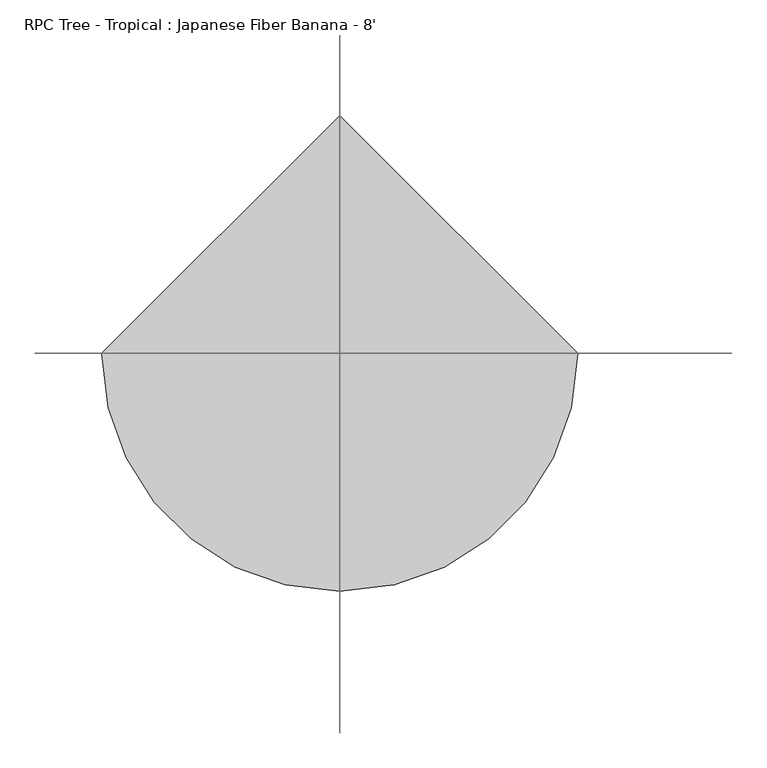
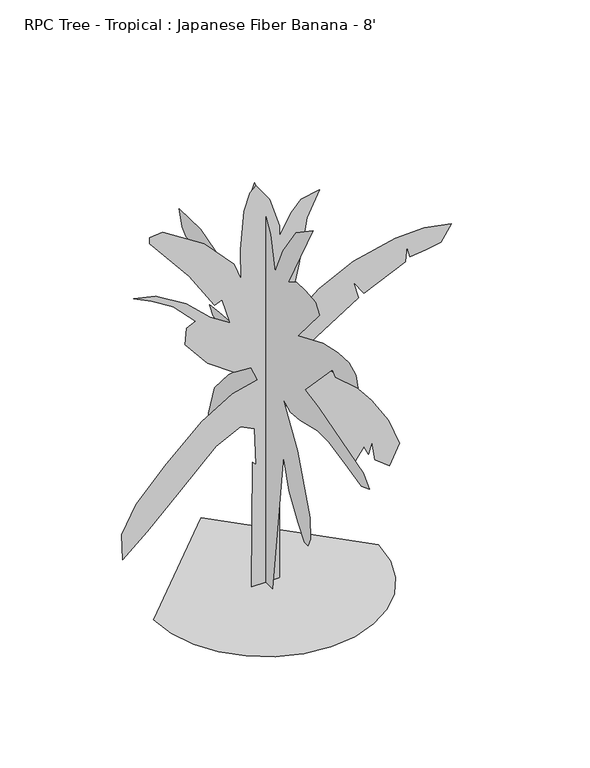
"""IFC4 building model written with IfcOpenShell, lengths in millimetres: geographic element geometry, RPC Tree - Tropical : Japanese Fiber Banana - 8'."""

from ifc_helpers import new_model, si_unit, origin, place, context, project, spatial, triangles, source, transform, mapped, element, save


def rpc_tree_tropical_japanese_fiber_banana_8_fc2fb2a9(model_context):
    return source(origin(), model_context, "Body", "Tessellation", [
        triangles([(-649.7467501, 0.0, 3.7e-06), (-632.5712723, -148.8792756, 3.7e-06), (-583.6506755, -285.6010629, 3.7e-06), (-506.9043426, -406.2488949, 3.7e-06), (-406.2488949, -506.9043426, 3.7e-06), (-285.6010629, -583.6506755, 3.7e-06), (-148.8792756, -632.5712723, 3.7e-06), (2.84e-05, -649.7467501, 3.7e-06), (148.8792756, -632.5712723, 3.7e-06), (285.6010629, -583.6506755, 3.7e-06), (406.2488949, -506.9043426, 3.7e-06), (506.9043426, -406.2488949, 3.7e-06), (583.6506755, -285.6010629, 3.7e-06), (632.5712723, -148.8790212, 3.7e-06), (649.7467501, 5.68e-05, 3.7e-06), (-8.52e-05, 649.7467501, 3.7e-06), (73.5169788, -2.4e-06, 1488.9400761), (86.1999983, -4e-06, 1501.9626823), (108.3956093, -6.3e-06, 1521.7797867), (138.5178168, -9.4e-06, 1547.2586094), (174.9816703, -1.3e-05, 1577.2688416), (216.2016834, -1.69e-05, 1610.6750874), (260.5921424, -2.12e-05, 1646.3444218), (306.5688237, -2.56e-05, 1683.149152), (505.0933339, -3.74e-05, 1782.4125698), (746.7776007, -4.41e-05, 1838.5162674), (915.0912369, -4.46e-05, 1842.831847), (1070.4584976, -4.1e-05, 1812.6209003), (1010.0392931, -3.02e-05, 1721.9908218), (923.7222507, -2.81e-05, 1704.7264687), (833.0921722, -2.71e-05, 1696.0954548), (815.8277464, -3.48e-05, 1760.832637), (807.1968052, -2.45e-05, 1674.5181381), (565.5150455, -1.17e-05, 1566.6237064), (505.0933339, -2.2e-05, 1652.9382053), (535.3041716, -9.6e-06, 1549.3592079), (250.4636001, 1.15e-05, 1372.4146305), (207.3058056, 2.02e-05, 1299.0465797), (457.6205775, 4.54e-05, 1087.573078), (608.672295, 6.81e-05, 897.679509), (707.9358582, 8.66e-05, 742.3123209), (772.6704969, 0.0001061, 578.3115755), (712.2512924, 0.00012, 461.7861663), (630.2496843, 0.0001123, 526.5233485), (612.9878019, 9.89e-05, 638.7333235), (591.4078691, 0.0001066, 573.9961049), (565.5150455, 0.0001, 630.1023823), (518.0422892, 0.0001082, 561.0496931), (237.5161527, 6.86e-05, 893.3640747), (99.411601, 4.9e-05, 1057.362204), (82.1486921, 4.08e-05, 1126.4148932), (77.8327038, 0.0001751, 0.0), (-81.8504909, 0.0001751, 0.0), (-77.5347659, 8.45e-05, 759.5742033), (-55.9558732, 8.71e-05, 737.996814), (-64.587582, 6.09e-05, 958.1012569), (-146.5871735, 5.57e-05, 1001.2585064), (-289.0071958, 6.39e-05, 932.2058172), (-500.4806794, 8.86e-05, 725.0478951), (-686.0587051, 0.0001097, 548.1032813), (-828.4769743, 0.0001241, 427.259858), (-832.7950247, 0.0001056, 582.6295896), (-750.7934166, 8.71e-05, 737.996814), (-573.8488029, 6.5e-05, 923.574876), (-371.0062786, 4.28e-05, 1109.1529381), (-194.0604295, 3e-05, 1217.044899), (-47.3244142, 2.59e-05, 1251.5712799), (-86.1662158, 1.56e-05, 1337.8882496), (-185.4289796, 1.46e-05, 1346.5192635), (-336.4799704, 1.7e-06, 1454.4136951), (-465.9543348, -1.73e-05, 1614.0963902), (-457.3233936, -2.87e-05, 1709.0419029), (-405.5326232, -3.18e-05, 1734.93727), (-535.0069877, -4.77e-05, 1868.7272141), (-660.1633381, -5.7e-05, 1946.4106991), (-763.7423355, -6.31e-05, 1998.1989624), (-638.583478, -5.95e-05, 1967.9881611), (-461.6388642, -4.67e-05, 1860.0962002), (-323.5335222, -3.12e-05, 1730.6218357), (-207.0078768, -2.25e-05, 1657.2536396), (-254.4808694, -4.1e-05, 1812.6209003), (-297.6381552, -3.9e-05, 1795.3590179), (-444.3744384, -6.62e-05, 2024.0943295), (-673.1097862, -9.91e-05, 2300.30247), (-673.1097862, -0.0001038, 2339.1442852), (-595.4261559, -0.0001043, 2343.4597195), (-358.0598668, -8.63e-05, 2192.4080383), (-185.4289796, -6.42e-05, 2006.8299763), (-142.2711851, -5.13e-05, 1898.9380154), (-146.5871735, -7.29e-05, 2080.198027), (-125.0082762, -0.0001002, 2308.9359547), (-90.4819498, -0.000112, 2408.1969017), (-55.9558732, -0.0001156, 2438.4078484), (21.7278389, -0.0001027, 2330.5132713), (77.8327038, -8.11e-05, 2149.2507889), (77.8327038, -7.39e-05, 2088.8315117), (146.8851113, -8.78e-05, 2205.3569572), (202.9900806, -9.5e-05, 2265.7760891), (310.8842943, -9.76e-05, 2287.3560219), (237.5161527, -8.01e-05, 2140.619775), (190.0426515, -4.87e-05, 1877.3580826), (142.5693864, -2.3e-05, 1661.5692192), (124.24932, -1.81e-05, 1620.2990639), (106.9864112, -1.34e-05, 1581.1042179), (91.8370452, -9.2e-06, 1546.0623161), (79.8586157, -5.8e-06, 1517.2485226), (72.1077807, -3.4e-06, 1496.740472), (69.6416885, -2.1e-06, 1486.6108578), (-6.07e-05, -228.3904198, 1972.5652073), (-6.46e-05, -305.2429235, 2016.4820034), (-6.49e-05, -396.7365758, 2020.139629), (-6.39e-05, -495.5454429, 2009.1616653), (-5.9e-05, -535.8019973, 1954.2670509), (-3.61e-05, -319.883527, 1698.0893738), (-4.56e-05, -568.7408298, 1804.2211224), (-4.86e-05, -718.786722, 1837.1573387), (-4.89e-05, -828.5760235, 1840.8175804), (-4.63e-05, -901.771483, 1811.5388443), (-4.01e-05, -920.0697121, 1742.0061699), (-3.38e-05, -696.8283966, 1672.4708794), (-3.65e-05, -667.5522039, 1701.7496155), (-1.06e-05, -393.0764068, 1412.635722), (-8.3e-06, -524.8241063, 1387.0172276), (3.5e-06, -974.9643265, 1255.2694553), (8.7e-06, -1037.1792789, 1196.7146719), (1.13e-05, -956.6660975, 1167.4360085), (8.7e-06, -821.2583015, 1196.7146719), (5.1e-06, -623.6354805, 1236.971299), (5.1e-06, -517.5038046, 1236.971299), (8.7e-06, -341.8393816, 1196.7146719), (9.7e-06, -246.688885, 1185.7342375), (6.4e-06, -169.8356182, 1222.3306229), (2.67e-05, -316.2233943, 995.4317545), (5.65e-05, -440.6507558, 662.4010649), (6.79e-05, -447.9710575, 534.3135707), (7.28e-05, -422.3525631, 479.4163765), (7.28e-05, -385.756105, 479.4163765), (6.53e-05, -323.5411526, 563.5896907), (5.32e-05, -232.0500619, 698.9975229), (3.75e-05, -177.1549025, 874.6619459), (5.84e-05, -147.8774926, 640.4427395), (0.0001157, -67.36457, 3.7e-06), (0.0001157, 82.6820898, 3.7e-06), (9.61e-05, 82.6820898, 219.5804016), (0.0001026, 64.3836201, 146.3870222), (7.84e-05, 35.1062147, 417.2039675), (4.99e-05, 35.1062147, 735.593981), (2.38e-05, 79.0221933, 1028.3680435), (2.8e-05, 174.1739435, 980.7936945), (4.14e-05, 331.5396469, 830.7452225), (5.19e-05, 430.3510211, 713.6355829), (5.84e-05, 444.9891174, 640.4427395), (5.58e-05, 470.6076118, 669.7214029), (6.33e-05, 466.9474792, 585.5480887), (6.01e-05, 529.1624316, 622.1445105), (6.5e-05, 551.1207933, 567.2498597), (5.45e-05, 573.0791914, 684.3594629), (3.75e-05, 514.5243716, 874.6619459), (2.28e-05, 375.4563704, 1039.3484779), (6.1e-06, 170.5143013, 1225.9908646), (1.8e-06, 272.9848271, 1273.567757), (-1.1e-06, 393.7545994, 1306.5039734), (2e-07, 459.6297209, 1291.8659134), (-1.1e-06, 529.1624316, 1306.5039734), (-5e-06, 565.7588533, 1350.4207695), (-6.4e-06, 466.9474792, 1365.0588295), (-7.7e-06, 254.6866163, 1379.6968895), (-1.32e-05, 331.5396469, 1441.911842), (-2.5e-05, 514.5243716, 1573.6594688), (-2.96e-05, 730.4453854, 1624.896603), (-2.96e-05, 799.9781324, 1624.896603), (-3.29e-05, 840.2346869, 1661.4929157), (-4.1e-05, 869.5133503, 1752.9841335), (-4.14e-05, 653.5923729, 1756.6442299), (-3.58e-05, 441.3289484, 1694.4292774), (-3.02e-05, 283.9652797, 1632.214325), (-1.62e-05, 108.2998484, 1474.8480583), (-5.35e-05, 152.215827, 1892.0520985), (-8.06e-05, 185.15287, 2195.804052), (-9.63e-05, 111.9594906, 2371.468475), (-9.01e-05, 46.0854001, 2301.9356552), (-7.67e-05, -45.4067079, 2151.889872), (-5.87e-05, -89.322691, 1950.6068092), (-7.44e-05, -169.8356182, 2126.2712322), (-9.14e-05, -301.5827909, 2316.5737152), (-0.0001016, -469.9294556, 2430.0231857)], [[15, 16, 1], [14, 15, 1], [14, 1, 2], [13, 14, 2], [13, 2, 3], [13, 3, 4], [12, 13, 4], [11, 12, 4], [11, 4, 5], [11, 5, 6], [11, 6, 7], [11, 7, 8], [11, 8, 9], [11, 9, 10], [75, 76, 77], [45, 46, 47], [53, 54, 55], [60, 61, 62], [98, 99, 100], [97, 98, 100], [27, 28, 29], [27, 29, 30], [47, 48, 49], [60, 62, 63], [59, 60, 63], [59, 63, 64], [58, 59, 64], [58, 64, 65], [74, 75, 77], [74, 77, 78], [73, 74, 78], [73, 78, 79], [42, 43, 44], [42, 44, 45], [41, 42, 45], [92, 93, 94], [91, 92, 94], [96, 97, 100], [96, 100, 101], [52, 53, 55], [51, 52, 55], [51, 55, 56], [57, 58, 65], [57, 65, 66], [57, 66, 67], [27, 30, 31], [27, 31, 32], [26, 27, 32], [84, 85, 86], [83, 84, 86], [83, 86, 87], [83, 87, 88], [82, 83, 88], [81, 82, 88], [81, 88, 89], [56, 57, 67], [51, 56, 67], [91, 94, 95], [90, 91, 95], [90, 95, 96], [89, 90, 96], [89, 96, 101], [89, 101, 102], [33, 34, 35], [32, 33, 35], [26, 32, 35], [25, 26, 35], [24, 25, 35], [81, 89, 102], [80, 81, 102], [80, 102, 103], [80, 103, 104], [80, 104, 105], [80, 105, 106], [80, 106, 107], [40, 41, 45], [40, 45, 47], [40, 47, 49], [39, 40, 49], [38, 39, 49], [38, 49, 50], [38, 50, 51], [38, 51, 67], [38, 67, 68], [35, 36, 37], [24, 35, 37], [23, 24, 37], [22, 23, 37], [21, 22, 37], [20, 21, 37], [19, 20, 37], [18, 19, 37], [17, 18, 37], [17, 37, 38], [17, 38, 68], [108, 17, 68], [80, 107, 108], [80, 108, 68], [80, 68, 69], [80, 69, 70], [80, 70, 71], [79, 80, 71], [73, 79, 71], [73, 71, 72], [143, 144, 145], [185, 186, 109], [184, 185, 109], [155, 156, 157], [183, 184, 109], [151, 152, 153], [153, 154, 155], [164, 165, 166], [163, 164, 166], [124, 125, 126], [179, 180, 181], [172, 173, 174], [171, 172, 174], [170, 171, 174], [169, 170, 174], [169, 174, 175], [142, 143, 145], [141, 142, 145], [141, 145, 146], [141, 146, 147], [140, 141, 147], [140, 147, 148], [162, 163, 166], [162, 166, 167], [161, 162, 167], [179, 181, 182], [178, 179, 182], [178, 182, 183], [153, 155, 157], [153, 157, 158], [151, 153, 158], [150, 151, 158], [150, 158, 159], [149, 150, 159], [149, 159, 160], [148, 149, 160], [124, 126, 127], [123, 124, 127], [123, 127, 128], [123, 128, 129], [118, 119, 120], [117, 118, 120], [116, 117, 120], [116, 120, 121], [115, 116, 121], [115, 121, 122], [114, 115, 122], [168, 169, 175], [168, 175, 176], [168, 176, 177], [167, 168, 177], [177, 178, 183], [122, 123, 129], [122, 129, 130], [112, 113, 114], [111, 112, 114], [110, 111, 114], [109, 110, 114], [183, 109, 114], [177, 183, 114], [177, 114, 122], [177, 122, 130], [177, 130, 131], [177, 131, 132], [167, 177, 132], [161, 167, 132], [160, 161, 132], [148, 160, 132], [140, 148, 132], [140, 132, 133], [140, 133, 134], [139, 140, 134], [138, 139, 134], [138, 134, 135], [137, 138, 135], [137, 135, 136]], closed=False),
    ])


if __name__ == "__main__":
    model = new_model("IFC4")
    model_context = context("Model", 3, world=origin())
    ifc_project = project(units=[si_unit("LENGTHUNIT", "METRE", prefix="MILLI")], contexts=[model_context])
    site = spatial("IfcSite", under=ifc_project)
    building = spatial("IfcBuilding", under=site)
    placement = place(None, origin())
    rpc_tree_tropical_japanese_fiber_banana_8_shape = rpc_tree_tropical_japanese_fiber_banana_8_fc2fb2a9(model_context)
    element("IfcGeographicElement", 1, ObjectType="RPC Tree - Tropical : Japanese Fiber Banana - 8'", at=placement, inside=building, context=model_context, shape_type="MappedRepresentation", body=[
        mapped(rpc_tree_tropical_japanese_fiber_banana_8_shape, transform((0.0, 0.0, 0.0), x_axis=(1.0, 0.0, 0.0), y_axis=(0.0, 1.0, 0.0), z_axis=(0.0, 0.0, 1.0))),
    ])
    save(model, "model.ifc")

# Revit data of these elements
# Type "RPC Tree - Tropical : Japanese Fiber Banana - 8'"
#   built-in parameter 1005198 = "{2, 15},{39, RPC-16-FVGT-NR7X-7G1M-A000-ST1L-LVER-AU},{1, 0},{1, 0},{2, 13},{1, 8},{5, Color},{1, 0},{1, 0},{3, 0.8},{3, 0.8},{3, 0.8},{1, 8},{7, BBoxMin},{1, 0},{1, 0},{1, 0},{1, 0},{1, 0},{1, 8},{7, BBoxMax},{1, 0},{1, 0},{1, 0},{1, 0},{1, 0},{2, 11},{9, RPCTypeId},{1, 0},{1, 0},{39, RPC-16-FVGT-NR7X-7G1M-A000-ST1L-LVER-AU},{1, 6},{14, RPCPlantHeight},{1, 0},{1, 0},{1, 8},{2, 11},{7, keyword},{1, 0},{1, 0},{35, :RPCs:Trees [Tropical]:Geometry:RPC},{2, 11},{8, category},{1, 0},{1, 0},{16, Trees [Tropical]},{2, 11},{12, LocalizedUID},{1, 0},{1, 0},{21, Japanese Fiber Banana},{2, 14},{6, Height},{1, 0},{1, 0},{1, 8},{1, 2},{16, Cast Reflections},{1, 0},{1, 0},{1, 0},{1, 2},{12, Cast Shadows},{1, 0},{1, 0},{1, 1},{1, 2},{9, Lock View},{1, 0},{1, 0},{1, 0},{1, 4},{5, ViewC},{1, 0},{1, 0},{1, 0},{21, assetlibrary_base.fbx},{1, 5},"
#   built-in parameter 1005195 = "RPC-16-FVGT-NR7X-7G1M-A000-ST1L-LVER-AU"
#   Type Comments = "Japanese Fiber Banana"
#   Assembly Code = "G2050500"
#   Height = 8' - 0"
#   Plan Symbol = element 387627
#   Default Elevation = 0
